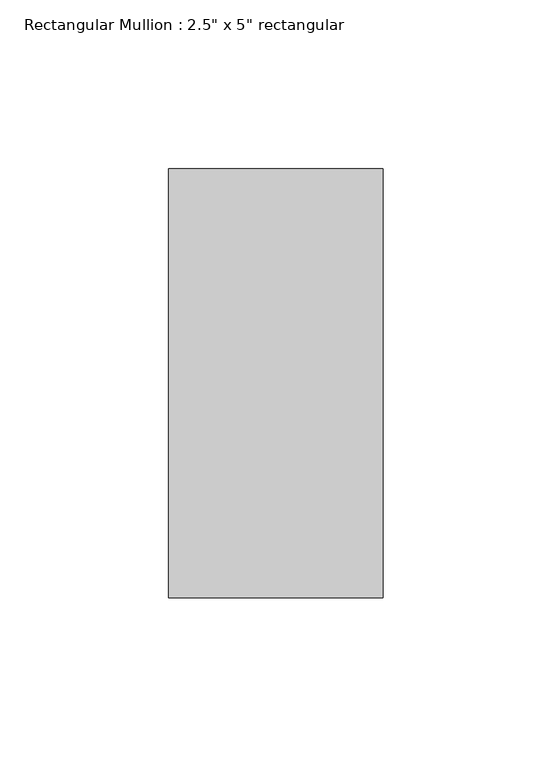
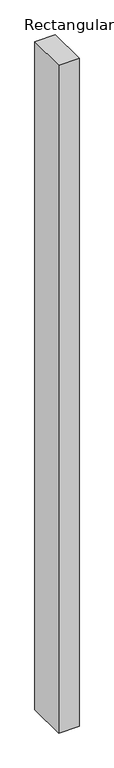
"""IFC4 building model written with IfcOpenShell, lengths in millimetres: member geometry."""

from ifc_helpers import new_model, si_unit, frame, origin, place, context, project, spatial, polyline, outline, extrude, source, transform, mapped, element, save


def member_8daf8b49(model_context):
    return source(origin(), model_context, "Body", "SweptSolid", [
        extrude(outline(polyline([(0.0, 63.5), (0.0, -63.5), (-63.5, -63.5), (-63.5, 63.5), (0.0, 63.5)])), frame((0.0, 0.0, -2190.75), z_axis=(0.0, 0.0, 1.0), x_axis=(1.0, 0.0, 0.0)), (0.0, 0.0, 1.0), 2190.75),
    ])


if __name__ == "__main__":
    model = new_model("IFC4")
    model_context = context("Model", 3, world=origin())
    ifc_project = project(units=[si_unit("LENGTHUNIT", "METRE", prefix="MILLI")], contexts=[model_context])
    site = spatial("IfcSite", under=ifc_project)
    building = spatial("IfcBuilding", under=site)
    placement = place(None, origin())
    member_shape = member_8daf8b49(model_context)
    element("IfcMember", 1, ObjectType="Rectangular Mullion : 2.5\" x 5\" rectangular", at=placement, inside=building, context=model_context, shape_type="MappedRepresentation", body=[
        mapped(member_shape, transform((0.0, 0.0, 0.0), x_axis=(1.0, 0.0, 0.0), y_axis=(0.0, 1.0, 0.0), z_axis=(0.0, 0.0, 1.0))),
    ])
    save(model, "model.ifc")

# Revit data of these elements
# Type "Rectangular Mullion : 2.5\" x 5\" rectangular"
#   built-in parameter 1007304 = 0.416667 (stored number, unit not read)
#   built-in parameter 1007301 = 0.104167 (stored number, unit not read)
#   built-in parameter 1007300 = 0.104167 (stored number, unit not read)
# Element 1 (IfcMember, "Rectangular Mullion : 2.5\" x 5\" rectangular")
#   Materials on its faces: "Iron, Ductile"
# Materials
#   "Iron, Ductile": class "Metal", colour RGB 0 0 0, transparency 0, Description = "Ductile cast iron", Cost = 0
